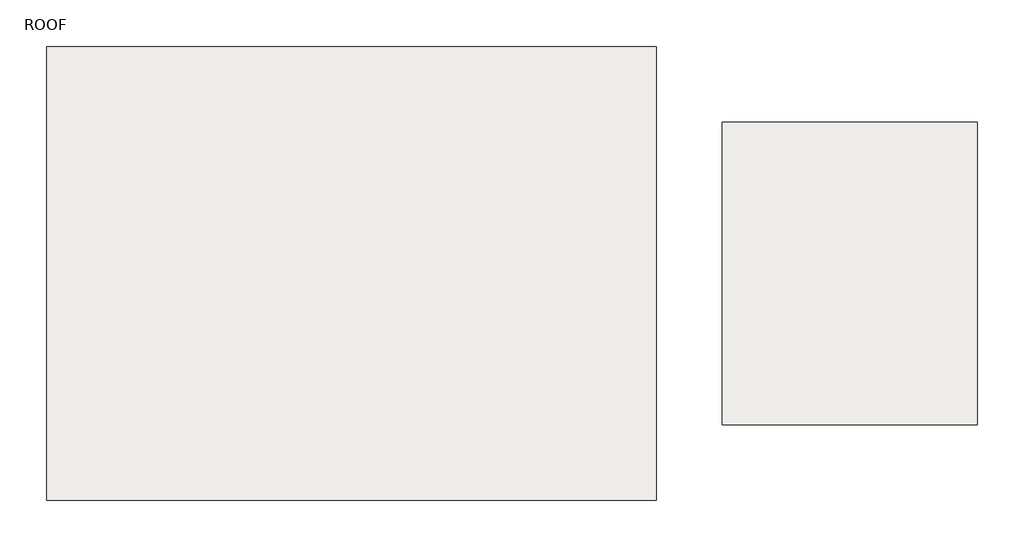
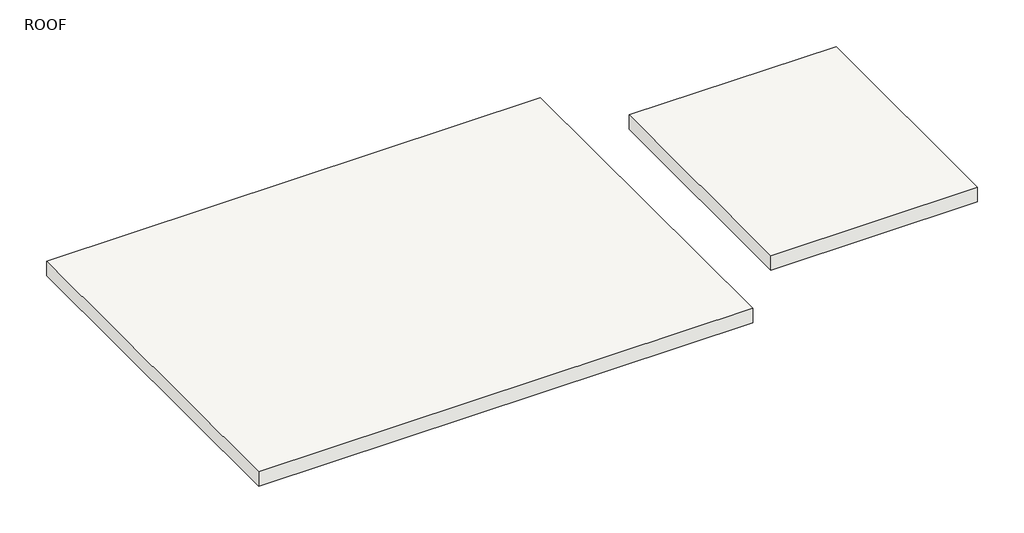
# One storey: 2 slabs.
"""IFC4 building model written with IfcOpenShell, lengths in millimetres."""

from ifc_helpers import new_model, si_unit, frame, origin, place, context, project, spatial, polyline, outline, extrude, element, save

model = new_model("IFC4")

# Units and contexts
model_context = context("Model", 3, world=origin())
ifc_project = project(units=[si_unit("LENGTHUNIT", "METRE", prefix="MILLI")], contexts=[model_context])

# Site, building, storey
site = spatial("IfcSite", under=ifc_project)
building = spatial("IfcBuilding", under=site)
storey = spatial("IfcBuildingStorey", under=building, Name="ROOF", Elevation=16002.0)

# Slabs
placement = place(None, origin())
element("IfcSlab", 1, ObjectType="6\"", at=placement, inside=storey, context=model_context, shape_type="SweptSolid", body=[
    extrude(outline(polyline([(-2052.9289041, 2388.0153263), (-2052.9289041, -1269.5846737), (-6967.8289041, -1269.5846737), (-6967.8289041, 2388.0153263), (-2052.9289041, 2388.0153263)])), frame((0.0, 0.0, 15849.6), z_axis=(0.0, 0.0, 1.0), x_axis=(1.0, 0.0, 0.0)), (0.0, 0.0, 1.0), 152.4),
])
element("IfcSlab", 2, ObjectType="6\"", at=placement, inside=storey, context=model_context, shape_type="SweptSolid", body=[
    extrude(outline(polyline([(537.8710959, 1778.4153263), (537.8710959, -659.9846737), (-1519.5289041, -659.9846737), (-1519.5289041, 1778.4153263), (537.8710959, 1778.4153263)])), frame((0.0, 0.0, 15849.6), z_axis=(0.0, 0.0, 1.0), x_axis=(1.0, 0.0, 0.0)), (0.0, 0.0, 1.0), 152.4),
])

save(model, "model.ifc")

# Revit data of these elements
# Type "6\""
#   Assembly Code = "B1010"
#   Function = 0
#   Layers, outside or top first: 0' - 6" no material (function 1)
# Elements 1, 2 (IfcSlab, "6\"")
#   Height Offset From Level = 0' - 0"
#   Phase Created = New Construction
#   Materials on its faces: "Default Floor", "DUSTY ROSE"
# Materials
#   "Default Floor": colour RGB 128 128 128, transparency 0, Cost = 0
#   "DUSTY ROSE": class "Generic", colour RGB 120 120 120, transparency 0, Cost = 0
